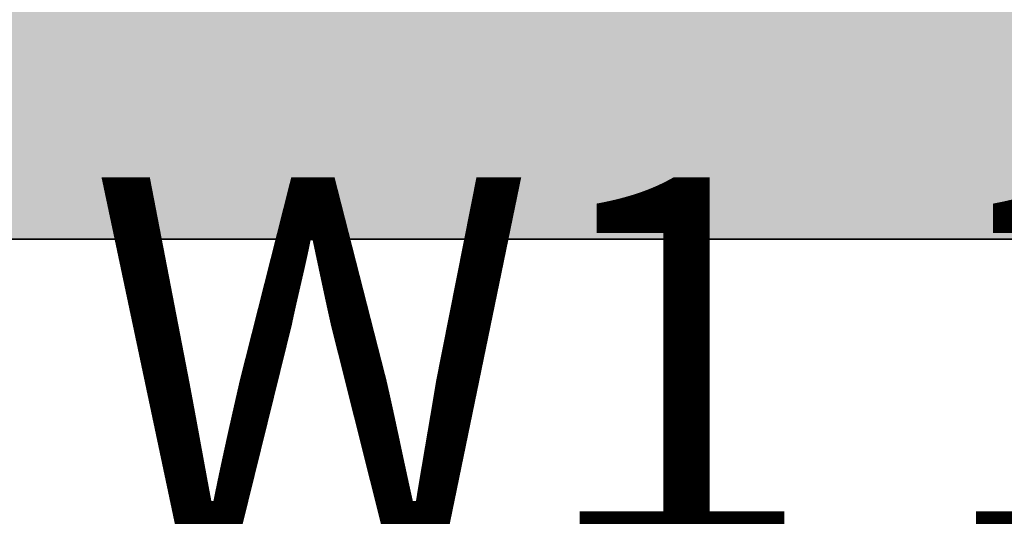
# Model space of a CAD drawing. Units: metres. Extents: x 4298.5 to 4325.2, y 2075 to 2095.8.
# Tile 8 of 35: x 4306.6693 to 4307.1445, y 2079.6943 to 2079.9341. Entities that reach past the tile are written whole.
import ezdxf

# ---------------------------------------------------------------- set-up
doc = ezdxf.new("R2010")
doc.units = ezdxf.units.M
for name, color, linetype, lineweight in [('A-ANNO-DIMS', 2, 'Continuous', 18), ('A-WALL', 7, 'Continuous', 35), ('A-WALL-PATT', 252, 'Continuous', 13)]:
    doc.layers.add(name, color=color, linetype=linetype, lineweight=lineweight)
doc.styles.get("Standard").update_dxf_attribs({"font": 'arial.ttf'})
doc.dimstyles.get("Standard").update_dxf_attribs({"dimtxt": 0.18, "dimasz": 0.18, "dimexe": 0.18, "dimexo": 0.0625, "dimgap": 0.09, "dimtad": 0, "dimtih": 1, "dimtoh": 1, "dimdec": 4, "dimzin": 0, "dimdsep": 46, "dimtxsty": 'Standard', "dimcen": 0.09, "dimadec": 0, "dimazin": 0, "dimtfac": 1, "dimtdec": 4, "dimtofl": 0, "dimtmove": 0, "dimatfit": 3, "dimfxl": 1, "dimtolj": 1, "dimtzin": 0, "dimarcsym": 0})

# ---------------------------------------------------------------- blocks, each defined once
blk = doc.blocks.new('*D23')
at = {"layer": 'A-ANNO-DIMS', "color": 0, "lineweight": -2, "transparency": 16777216}
for p, q in [((4308.16058, 2079.85556), (4308.16058, 2079.58806)), ((4309.16058, 2079.85556), (4309.16058, 2079.58806)), ((4308.16058, 2079.76806), (4307.98058, 2079.76806)), ((4308.98058, 2079.76806), (4308.34058, 2079.76806))]:
    blk.add_line(p, q, dxfattribs=at)
at = {"layer": 'A-ANNO-DIMS', "color": 0, "transparency": 16777216}
for points in [[(4308.34058, 2079.79806), (4308.34058, 2079.73806), (4308.16058, 2079.76806)], [(4308.98058, 2079.79806), (4308.98058, 2079.73806), (4309.16058, 2079.76806)]]:
    blk.add_solid(points, dxfattribs=at)
at = {"layer": 'Defpoints', "color": 0, "transparency": 16777216}
for p in [(4308.16058, 2079.91806), (4309.16058, 2079.91806), (4308.16058, 2079.76806)]:
    blk.add_point(p, dxfattribs=at)
at = {"layer": 'A-ANNO-DIMS', "color": 0, "transparency": 16777216, "insert": (4306.70861, 2079.76806), "char_height": 0.18, "attachment_point": 5}
blk.add_mtext('\\A1;WINDOW W1 1 TYP.', dxfattribs=at)
blk = doc.blocks.new('*D47')
at = {"layer": 'A-ANNO-DIMS', "color": 0, "lineweight": -2, "transparency": 16777216}
for p, q in [((4300.43058, 2084.49556), (4300.43058, 2074.98956)), ((4322.81058, 2084.49556), (4322.81058, 2074.98956)), ((4300.61058, 2075.16956), (4311.22515, 2075.16956)), ((4322.63058, 2075.16956), (4312.016, 2075.16956))]:
    blk.add_line(p, q, dxfattribs=at)
at = {"layer": 'A-ANNO-DIMS', "color": 0, "transparency": 16777216}
for points in [[(4300.61058, 2075.19956), (4300.61058, 2075.13956), (4300.43058, 2075.16956)], [(4322.63058, 2075.19956), (4322.63058, 2075.13956), (4322.81058, 2075.16956)]]:
    blk.add_solid(points, dxfattribs=at)
at = {"layer": 'Defpoints', "color": 0, "transparency": 16777216}
for p in [(4300.43058, 2084.55806), (4322.81058, 2084.55806), (4322.81058, 2075.16956)]:
    blk.add_point(p, dxfattribs=at)
at = {"layer": 'A-ANNO-DIMS', "color": 0, "transparency": 16777216, "insert": (4311.62058, 2075.16956), "char_height": 0.18, "attachment_point": 5}
blk.add_mtext('\\A1;22.38', dxfattribs=at)
blk = doc.blocks.new('*D54')
at = {"layer": 'A-ANNO-DIMS', "color": 0, "lineweight": -2, "transparency": 16777216}
for p, q in [((4305.59808, 2079.82806), (4299.09208, 2079.82806)), ((4299.27208, 2079.64806), (4299.27208, 2078.26002)), ((4299.27208, 2076.50806), (4299.27208, 2077.89609)), ((4309.09808, 2076.32806), (4299.09208, 2076.32806))]:
    blk.add_line(p, q, dxfattribs=at)
at = {"layer": 'A-ANNO-DIMS', "color": 0, "transparency": 16777216}
for points in [[(4299.24208, 2079.64806), (4299.30208, 2079.64806), (4299.27208, 2079.82806)], [(4299.24208, 2076.50806), (4299.30208, 2076.50806), (4299.27208, 2076.32806)]]:
    blk.add_solid(points, dxfattribs=at)
at = {"layer": 'Defpoints', "color": 0, "transparency": 16777216}
for p in [(4305.66058, 2079.82806), (4299.27208, 2076.32806), (4309.16058, 2076.32806)]:
    blk.add_point(p, dxfattribs=at)
at = {"layer": 'A-ANNO-DIMS', "color": 0, "transparency": 16777216, "insert": (4299.27208, 2078.07806), "char_height": 0.18, "attachment_point": 5}
blk.add_mtext('\\A1;3.5', dxfattribs=at)
blk = doc.blocks.new('*D59')
at = {"layer": 'A-ANNO-DIMS', "color": 0, "lineweight": -2, "transparency": 16777216}
for p, q in [((4305.89058, 2079.99556), (4305.89058, 2074.98956)), ((4307.39058, 2079.99556), (4307.39058, 2074.98956)), ((4306.07058, 2075.16956), (4306.39452, 2075.16956)), ((4307.21058, 2075.16956), (4306.88663, 2075.16956))]:
    blk.add_line(p, q, dxfattribs=at)
at = {"layer": 'A-ANNO-DIMS', "color": 0, "transparency": 16777216}
for points in [[(4306.07058, 2075.19956), (4306.07058, 2075.13956), (4305.89058, 2075.16956)], [(4307.21058, 2075.19956), (4307.21058, 2075.13956), (4307.39058, 2075.16956)]]:
    blk.add_solid(points, dxfattribs=at)
at = {"layer": 'Defpoints', "color": 0, "transparency": 16777216}
for p in [(4305.89058, 2080.05806), (4307.39058, 2080.05806), (4307.39058, 2075.16956)]:
    blk.add_point(p, dxfattribs=at)
at = {"layer": 'A-ANNO-DIMS', "color": 0, "transparency": 16777216, "insert": (4306.64058, 2075.16956), "char_height": 0.18, "attachment_point": 5}
blk.add_mtext('\\A1;1.5', dxfattribs=at)
blk = doc.blocks.new('*D78')
at = {"layer": 'A-ANNO-DIMS', "color": 0, "lineweight": -2, "transparency": 16777216}
for p, q in [((4312.4969, 2079.73934), (4312.4969, 2079.91934)), ((4312.4069, 2079.82934), (4312.5869, 2079.82934)), ((4305.38467, 2076.78063), (4307.88631, 2077.85298)), ((4305.20467, 2076.78063), (4305.38467, 2076.78063))]:
    blk.add_line(p, q, dxfattribs=at)
at = {"layer": 'A-ANNO-DIMS', "color": 0, "transparency": 16777216}
blk.add_solid([(4307.87449, 2077.88055), (4307.89813, 2077.8254), (4308.05176, 2077.92389)], dxfattribs=at)
at = {"layer": 'Defpoints', "color": 0, "transparency": 16777216}
for p in [(4312.4969, 2079.82934), (4308.05176, 2077.92389)]:
    blk.add_point(p, dxfattribs=at)
at = {"layer": 'A-ANNO-DIMS', "color": 0, "transparency": 16777216, "insert": (4304.52998, 2076.78063), "char_height": 0.18, "attachment_point": 5}
blk.add_mtext('\\A1;2X R4.836', dxfattribs=at)

msp = doc.modelspace()

# ---------------------------------------------------------------- hatches: boundary and pattern name
at = {"layer": 'A-WALL-PATT'}
h = msp.add_hatch(color=256, dxfattribs=at)
h.dxf.hatch_style = 1
h.paths.add_polyline_path([(4308.76058, 2094.47806), (4308.16058, 2094.47806), (4307.46058, 2094.47806), (4307.46058, 2094.24806), (4308.27058, 2094.24806), (4308.27058, 2094.12806), (4308.39058, 2094.12806), (4308.39058, 2094.24806), (4308.76058, 2094.24806)])
h.paths.add_polyline_path([(4310.12058, 2094.47806), (4309.52058, 2094.47806), (4309.52058, 2094.24806), (4309.89058, 2094.24806), (4309.89058, 2092.24806), (4308.39058, 2092.24806), (4308.39058, 2093.42806), (4308.27058, 2093.42806), (4308.27058, 2092.01806), (4309.89058, 2092.01806), (4309.89058, 2087.01806), (4309.77058, 2087.01806), (4309.77058, 2086.78806), (4309.89058, 2086.78806), (4311.94058, 2086.78806), (4311.94058, 2087.01806), (4310.12058, 2087.01806), (4310.12058, 2089.01806), (4310.24058, 2089.01806), (4310.24058, 2089.13806), (4310.12058, 2089.13806), (4310.12058, 2092.01806), (4310.30785, 2092.01806), (4310.30785, 2092.24806), (4310.12058, 2092.24806)])
h.paths.add_polyline_path([(4311.74058, 2092.24806), (4311.06785, 2092.24806), (4311.06785, 2092.01806), (4311.74058, 2092.01806)], flags=17)
h.paths.add_polyline_path([(4313.17331, 2092.24806), (4312.50058, 2092.24806), (4312.50058, 2092.01806), (4313.17331, 2092.01806)])
h.paths.add_polyline_path([(4314.53785, 2092.24806), (4314.12058, 2092.24806), (4313.93331, 2092.24806), (4313.93331, 2092.01806), (4314.12058, 2092.01806), (4314.12058, 2087.01806), (4314.00058, 2087.01806), (4314.00058, 2086.78806), (4314.12058, 2086.78806), (4315.57179, 2086.78806), (4315.57179, 2087.01806), (4314.35058, 2087.01806), (4314.35058, 2092.01806), (4314.53785, 2092.01806)])
h.paths.add_polyline_path([(4315.97058, 2092.24806), (4315.29785, 2092.24806), (4315.29785, 2092.01806), (4315.97058, 2092.01806)])
h.paths.add_polyline_path([(4317.40331, 2092.24806), (4316.73058, 2092.24806), (4316.73058, 2092.01806), (4317.40331, 2092.01806)])
h.paths.add_polyline_path([(4318.95058, 2092.24806), (4318.35058, 2092.24806), (4318.16331, 2092.24806), (4318.16331, 2092.01806), (4318.35058, 2092.01806), (4318.35058, 2091.89806), (4318.58058, 2091.89806), (4318.58058, 2092.01806), (4318.95058, 2092.01806)])
h.paths.add_polyline_path([(4321.01058, 2092.24806), (4319.71058, 2092.24806), (4319.71058, 2092.01806), (4320.08058, 2092.01806), (4320.08058, 2090.01806), (4318.58058, 2090.01806), (4318.58058, 2091.19806), (4318.35058, 2091.19806), (4318.35058, 2090.01806), (4318.35058, 2087.01806), (4318.23058, 2087.01806), (4318.23058, 2086.78806), (4318.35058, 2086.78806), (4318.35058, 2086.30806), (4318.58058, 2086.30806), (4318.58058, 2089.78806), (4321.78058, 2089.78806), (4321.78058, 2090.01806), (4320.20058, 2090.01806), (4320.20058, 2092.01806), (4321.01058, 2092.01806)])
h.paths.add_polyline_path([(4322.81058, 2092.24806), (4321.77058, 2092.24806), (4321.77058, 2092.01806), (4322.58058, 2092.01806), (4322.58058, 2091.28306), (4322.81058, 2091.28306)])
h.paths.add_polyline_path([(4322.81058, 2090.52306), (4322.58058, 2090.52306), (4322.58058, 2089.78806), (4322.58058, 2089.52545), (4322.81058, 2089.52545), (4322.81058, 2090.01806)])
h.paths.add_polyline_path([(4322.81058, 2088.76545), (4322.58058, 2088.76545), (4322.58058, 2087.66806), (4322.81058, 2087.66806)])
h.paths.add_polyline_path([(4322.81058, 2086.90806), (4322.58058, 2086.90806), (4322.58058, 2085.81066), (4322.81058, 2085.81066)])
h.paths.add_polyline_path([(4322.81058, 2085.05066), (4322.58058, 2085.05066), (4322.58058, 2084.78806), (4318.58058, 2084.78806), (4318.58058, 2085.05806), (4318.58058, 2085.40806), (4318.35058, 2085.40806), (4318.35058, 2084.55806), (4318.35058, 2080.85806), (4318.47058, 2080.85806), (4318.47058, 2082.32806), (4319.26058, 2082.32806), (4319.26058, 2082.55806), (4318.58058, 2082.55806), (4318.58058, 2084.55806), (4320.08058, 2084.55806), (4320.08058, 2083.93806), (4320.31058, 2083.93806), (4320.31058, 2084.55806), (4322.81058, 2084.55806)])
h.paths.add_polyline_path([(4320.31058, 2083.17806), (4320.08058, 2083.17806), (4320.08058, 2082.55806), (4319.96058, 2082.55806), (4319.96058, 2082.32806), (4320.08058, 2082.32806), (4320.08058, 2081.57306), (4320.31058, 2081.57306)], flags=17)
h.paths.add_polyline_path([(4320.31058, 2080.81306), (4320.08058, 2080.81306), (4320.08058, 2080.05806), (4318.42861, 2080.05806), (4318.42861, 2079.82806), (4320.31058, 2079.82806)])
h.paths.add_polyline_path([(4317.35058, 2085.28806), (4316.57179, 2085.28806), (4316.57179, 2085.05806), (4317.35058, 2085.05806)])
h.paths.add_polyline_path([(4315.57179, 2085.28806), (4314.84342, 2085.28806), (4314.84342, 2085.05806), (4315.57179, 2085.05806)])
h.paths.add_polyline_path([(4313.84342, 2085.28806), (4312.94058, 2085.28806), (4312.94058, 2085.05806), (4313.84342, 2085.05806)])
h.paths.add_polyline_path([(4311.94058, 2085.28806), (4311.44058, 2085.28806), (4311.44058, 2085.05806), (4311.94058, 2085.05806)])
h.paths.add_polyline_path([(4317.33058, 2087.01806), (4316.57179, 2087.01806), (4316.57179, 2086.78806), (4317.33058, 2086.78806)])
h.paths.add_polyline_path([(4313.10058, 2089.13806), (4311.14058, 2089.13806), (4311.14058, 2089.01806), (4312.98058, 2089.01806), (4312.98058, 2087.01806), (4312.94058, 2087.01806), (4312.94058, 2086.78806), (4313.10058, 2086.78806), (4313.10058, 2087.01806)])
h.paths.add_polyline_path([(4307.55152, 2087.01806), (4305.89058, 2087.01806), (4305.89058, 2092.24806), (4305.89058, 2094.24806), (4306.70058, 2094.24806), (4306.70058, 2094.47806), (4305.66058, 2094.47806), (4305.66058, 2092.24806), (4305.29058, 2092.24806), (4305.29058, 2092.01806), (4305.66058, 2092.01806), (4305.66058, 2090.01806), (4304.16058, 2090.01806), (4304.16058, 2091.19806), (4304.04058, 2091.19806), (4304.04058, 2089.90806), (4301.56058, 2089.90806), (4301.56058, 2089.78806), (4304.04058, 2089.78806), (4305.66058, 2089.78806), (4305.66058, 2086.63806), (4305.89058, 2086.63806), (4305.89058, 2086.78806), (4307.55152, 2086.78806)])
h.paths.add_polyline_path([(4307.55152, 2085.28806), (4305.89058, 2085.28806), (4305.89058, 2085.43806), (4305.66058, 2085.43806), (4305.66058, 2084.78806), (4305.29058, 2084.78806), (4305.29058, 2084.55806), (4305.66058, 2084.55806), (4305.66058, 2084.02001), (4305.89058, 2084.02001), (4305.89058, 2084.55806), (4305.89058, 2085.05806), (4307.55152, 2085.05806)])
h.paths.add_polyline_path([(4310.24058, 2085.28806), (4308.55152, 2085.28806), (4308.55152, 2085.05806), (4310.24058, 2085.05806)])
h.paths.add_polyline_path([(4317.42861, 2080.05806), (4316.57179, 2080.05806), (4316.57179, 2079.82806), (4317.42861, 2079.82806)])
h.paths.add_polyline_path([(4315.57179, 2080.05806), (4314.84342, 2080.05806), (4314.84342, 2079.82806), (4315.57179, 2079.82806)])
h.paths.add_polyline_path([(4313.84342, 2080.05806), (4312.94058, 2080.05806), (4312.94058, 2079.82806), (4313.84342, 2079.82806)])
h.paths.add_polyline_path([(4311.94058, 2080.05806), (4311.44058, 2080.05806), (4311.44058, 2079.82806), (4311.94058, 2079.82806)])
h.paths.add_polyline_path([(4310.24058, 2080.05806), (4310.12058, 2080.05806), (4310.12058, 2084.03806), (4309.89058, 2084.03806), (4309.89058, 2080.05806), (4309.16058, 2080.05806), (4309.16058, 2079.82806), (4310.24058, 2079.82806)])
h.paths.add_polyline_path([(4308.16058, 2080.05806), (4307.51058, 2080.05806), (4307.51058, 2080.17806), (4307.39058, 2080.17806), (4307.39058, 2080.05806), (4305.89058, 2080.05806), (4305.89058, 2080.56697), (4305.66058, 2080.56697), (4305.66058, 2079.82806), (4308.16058, 2079.82806)])
h.paths.add_polyline_path([(4307.51058, 2081.93806), (4309.09058, 2081.93806), (4309.09058, 2082.05806), (4305.89058, 2082.05806), (4305.89058, 2083.26001), (4305.66058, 2083.26001), (4305.66058, 2081.32697), (4305.89058, 2081.32697), (4305.89058, 2081.93806), (4307.39058, 2081.93806), (4307.39058, 2080.87806), (4307.51058, 2080.87806)])
h.paths.add_polyline_path([(4304.53058, 2084.78806), (4302.73058, 2084.78806), (4302.73058, 2084.55806), (4304.53058, 2084.55806)])
h.paths.add_polyline_path([(4301.97058, 2084.78806), (4300.66058, 2084.78806), (4300.66058, 2085.02492), (4300.43058, 2085.02492), (4300.43058, 2084.55806), (4301.97058, 2084.55806)])
h.paths.add_polyline_path([(4300.66058, 2086.88429), (4300.43058, 2086.88429), (4300.43058, 2085.78492), (4300.66058, 2085.78492)])
h.paths.add_polyline_path([(4300.66058, 2089.16182), (4300.43058, 2089.16182), (4300.43058, 2087.64429), (4300.66058, 2087.64429)])
h.paths.add_polyline_path([(4300.66058, 2091.02119), (4300.43058, 2091.02119), (4300.43058, 2089.92182), (4300.66058, 2089.92182)])
h.paths.add_polyline_path([(4300.66058, 2092.01806), (4301.97058, 2092.01806), (4301.97058, 2092.24806), (4300.43058, 2092.24806), (4300.43058, 2091.78119), (4300.66058, 2091.78119)])
h.paths.add_polyline_path([(4304.53058, 2092.24806), (4302.73058, 2092.24806), (4302.73058, 2092.01806), (4304.04058, 2092.01806), (4304.04058, 2091.89806), (4304.16058, 2091.89806), (4304.16058, 2092.01806), (4304.53058, 2092.01806)], flags=17)

# ---------------------------------------------------------------- linework, layer by layer
at = {"layer": 'A-WALL'}
msp.add_line((4310.24058, 2079.82806), (4305.66058, 2079.82806), dxfattribs=at)

# ---------------------------------------------------------------- dimensions: what is measured, and where the dimension line sits
at = {"layer": 'A-ANNO-DIMS'}
for base, p1, p2, override, picture, middle in [((4322.81058, 2075.16956), (4300.43058, 2084.55806), (4322.81058, 2084.55806), {"dimdec": 2, "dimlfac": 1, "dimrnd": 0, "dimzin": 0, "dimdsep": 46, "dimlunit": 2}, '*D47', (4311.62058, 2075.16956)), ((4307.39058, 2075.16956), (4305.89058, 2080.05806), (4307.39058, 2080.05806), {"dimdec": 1, "dimlfac": 1, "dimrnd": 0, "dimzin": 0, "dimdsep": 46, "dimlunit": 2}, '*D59', (4306.64058, 2075.16956))]:
    dim = msp.add_linear_dim(base=base, p1=p1, p2=p2, dimstyle='Standard', override=override, dxfattribs=at)
    dim.commit()
    dim.dimension.update_dxf_attribs({"geometry": picture, "text_midpoint": middle})
dim = msp.add_linear_dim(base=(4308.16058, 2079.76806), p1=(4309.16058, 2079.91806), p2=(4308.16058, 2079.91806), angle=180, text='WINDOW W1 <> TYP.', dimstyle='Standard', override={"dimdec": 0, "dimlfac": 1, "dimrnd": 0, "dimzin": 0, "dimdsep": 46, "dimlunit": 2}, dxfattribs=at)
dim.commit()
dim.dimension.update_dxf_attribs({"geometry": '*D23', "text_midpoint": (4306.70861, 2079.76806)})
dim = msp.add_radius_dim(center=(4312.4969, 2079.82934), mpoint=(4308.05176, 2077.92389), text='2X <>', dimstyle='Standard', override={"dimdec": 3, "dimlfac": 1, "dimrnd": 0, "dimzin": 0, "dimdsep": 46, "dimlunit": 2}, dxfattribs=at)
dim.commit()
dim.dimension.update_dxf_attribs({"geometry": '*D78', "text_midpoint": (4304.52998, 2076.78063), "dimtype": 164})
dim = msp.add_linear_dim(base=(4299.27208, 2076.32806), p1=(4305.66058, 2079.82806), p2=(4309.16058, 2076.32806), angle=90, dimstyle='Standard', override={"dimdec": 1, "dimlfac": 1, "dimrnd": 0, "dimzin": 0, "dimdsep": 46, "dimlunit": 2}, dxfattribs=at)
dim.commit()
dim.dimension.update_dxf_attribs({"geometry": '*D54', "text_midpoint": (4299.27208, 2078.07806)})

doc.saveas('drawing.dxf')
